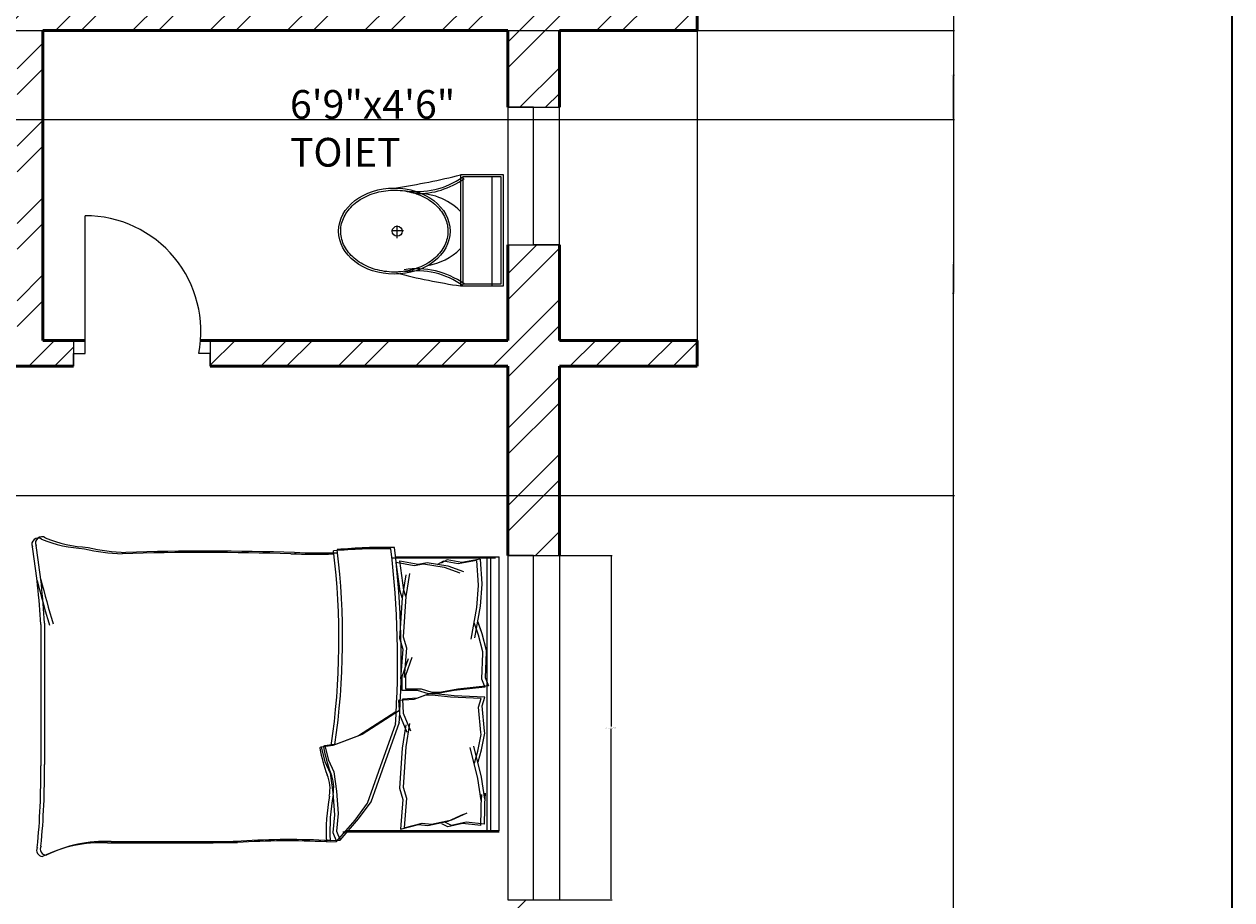
# Model space of a CAD drawing. Units: inches. Extents: x 1980 to 2738, y 1471 to 2568.
# Tile 13 of 22: x 2528 to 2738, y 1722 to 1874. Entities that reach past the tile are written whole.
import ezdxf

# ---------------------------------------------------------------- set-up
doc = ezdxf.new("R2010")
doc.units = ezdxf.units.IN
for name, color, linetype, lineweight in [('A-ANNO-DIMS', 2, 'Continuous', 18), ('A-ANNO-TTLB', 7, 'Continuous', 35), ('A-AREA-IDEN', 7, 'Continuous', 18), ('A-DOOR', 31, 'Continuous', 25), ('A-FLOR-BALC', 7, 'Continuous', 25), ('A-FLOR-FIXT', 8, 'Continuous', 25), ('A-FURN', 8, 'Continuous', 18), ('A-GLAZ', 141, 'Continuous', 18), ('A-WALL', 7, 'Continuous', 50)]:
    doc.layers.add(name, color=color, linetype=linetype, lineweight=lineweight)
doc.layers.add('A-WALL-PATT', color=9, linetype='Continuous', lineweight=13, true_color=0xd19cc7)
doc.styles.get("Standard").update_dxf_attribs({"font": 'arial.ttf'})
doc.dimstyles.get("Standard").update_dxf_attribs({"dimtxt": 0.18, "dimasz": 0.18, "dimexe": 0.18, "dimexo": 0.0625, "dimgap": 0.09, "dimtad": 0, "dimtih": 1, "dimtoh": 1, "dimdec": 4, "dimzin": 0, "dimdsep": 46, "dimtxsty": 'Standard', "dimcen": 0.09, "dimadec": 0, "dimazin": 0, "dimtfac": 1, "dimtdec": 4, "dimtofl": 0, "dimtmove": 0, "dimatfit": 3, "dimfxl": 1, "dimtolj": 1, "dimtzin": 0, "dimarcsym": 0})

# ---------------------------------------------------------------- blocks, each defined once
blk = doc.blocks.new('A$C31115884')
for p, q in [((257.5, 466.4), (257.5, 523.2)), ((283.1, 497.7), (223.4, 497.7)), ((0, 200), (0, 0)), ((520, 200), (0, 200)), ((10, 190), (10, 10)), ((510, 190), (10, 190)), ((510, 10), (510, 190)), ((520, 0), (520, 200)), ((510, 54.5), (0, 54.5)), ((10, 10), (510, 10)), ((0, 0), (520, 0))]:
    blk.add_line(p, q)
blk.add_circle((255.6, 496.4), 23.6)
for centre, radius, start, end in [((2777.7, -204.6), 2807, 165.4549, 171.7133), ((-294.5, 403.3), 364.7, 324.2091, 9.3499), ((-294.5, 403.3), 374.7, 324.2091, 9.3499), ((805.8, 403.3), 364.7, 170.6501, 215.7909), ((3237, 905), 2807, 188.2867, 194.5451), ((139.5, 406.2), 293.5, 315.8436, 2.6563), ((805.8, 403.3), 374.7, 179.2036, 215.7909), ((383.6, 406.2), 293.5, 190.2774, 224.1564)]:
    blk.add_arc(centre, radius, start, end)
blk.add_ellipse((256.2, 509.9), major_axis=(0, -260.7), ratio=0.772727)
blk.add_open_spline([(256.2, 259.2), (263.1, 259.2), (270, 259.7), (287.8, 262.3), (298.7, 265.1), (319.9, 273.1), (330.2, 278.4), (350.1, 291.1), (359.7, 298.7), (377.7, 315.9), (386.2, 325.5), (401.7, 346.6), (408.8, 358.1), (421.3, 382.5), (426.8, 395.5), (435.9, 422.4), (439.5, 436.4), (444.8, 465.1), (446.5, 479.7), (447.9, 509.2), (447.6, 524), (445, 553.3), (442.7, 567.8), (436.3, 596), (432.1, 609.7), (421.9, 636), (416, 648.6), (402.5, 672.1), (395, 683), (378.6, 703), (369.8, 712.1), (351.1, 728), (341.3, 734.8), (320.9, 746.2), (310.4, 750.7), (288.9, 757.3), (278, 759.4), (256, 761), (245, 760.6), (223.1, 757.2), (212.3, 754.3), (191.1, 746.1), (180.8, 740.7), (160.9, 727.8), (151.4, 720.1), (133.5, 702.7), (125.1, 693), (109.6, 671.7), (102.6, 660.2), (90.2, 635.7), (84.9, 622.7), (76, 595.6), (72.4, 581.6), (67.2, 552.9), (65.6, 538.2), (64.4, 508.8), (64.8, 494), (67.5, 464.7), (69.9, 450.2), (76.6, 422), (80.8, 408.3), (91.1, 382.2), (97.2, 369.7), (110.8, 346.3), (118.4, 335.4), (134.8, 315.6), (143.7, 306.7), (162.4, 290.9), (172.3, 284.2), (192.8, 273), (203.3, 268.6), (224.8, 262.2), (235.8, 260.2), (249.9, 259.3), (253, 259.2), (256.2, 259.2)], degree=3, knots=[0, 0, 0, 0, 0.110105, 0.110105, 0.285049, 0.285049, 0.459994, 0.459994, 0.634938, 0.634938, 0.809882, 0.809882, 0.984827, 0.984827, 1.159771, 1.159771, 1.334715, 1.334715, 1.50966, 1.50966, 1.684604, 1.684604, 1.859549, 1.859549, 2.034493, 2.034493, 2.209437, 2.209437, 2.384382, 2.384382, 2.559326, 2.559326, 2.73427, 2.73427, 2.909215, 2.909215, 3.084159, 3.084159, 3.259103, 3.259103, 3.434048, 3.434048, 3.608992, 3.608992, 3.783936, 3.783936, 3.958881, 3.958881, 4.133825, 4.133825, 4.30877, 4.30877, 4.483714, 4.483714, 4.658658, 4.658658, 4.833603, 4.833603, 5.008547, 5.008547, 5.183491, 5.183491, 5.358436, 5.358436, 5.53338, 5.53338, 5.708324, 5.708324, 5.883269, 5.883269, 6.058213, 6.058213, 6.233158, 6.233158, 6.283185, 6.283185, 6.283185, 6.283185])
blk = doc.blocks.new('BED-DOUBLE')
for p, q in [((27.75, 52.87), (24.5, 49.16)), ((27.75, 52.87), (24.5, 49.16)), ((28.38, 53.1), (25.13, 49.39)), ((28.38, 53.1), (25.13, 49.39)), ((29.49, 52.95), (27.75, 52.87, 3.87)), ((29.49, 52.95), (27.75, 52.87, 3.87)), ((28.36, 51.33), (27.75, 52.87)), ((28.36, 51.33), (27.75, 52.87)), ((30.13, 53.18), (28.38, 53.1, 3.87)), ((30.13, 53.18), (28.38, 53.1, 3.87)), ((29, 51.56), (28.38, 53.1)), ((29, 51.56), (28.38, 53.1)), ((0, 51.49), (0.64, 51.49)), ((0, 51.27), (26.61, 51.27)), ((0, 51.27), (26.61, 51.27)), ((0, 51.27), (0, 3.48)), ((0.64, 51.49), (27.25, 51.49)), ((0.64, 51.49), (27.25, 51.49)), ((1.53, 3.48), (1.53, 51.27)), ((1.53, 3.48), (1.53, 51.27)), ((2.17, 3.7), (2.17, 51.49)), ((2.17, 3.7), (2.17, 51.49)), ((6.41, 49.96), (8.98, 50.56)), ((6.41, 49.96), (8.98, 50.56)), ((8.98, 50.56), (10.02, 50.04)), ((8.98, 50.56), (10.02, 50.04)), ((16.57, 50.7), (13.43, 49.92)), ((16.57, 50.7), (13.43, 49.92)), ((17.21, 50.93), (14.07, 50.15)), ((17.21, 50.93), (14.07, 50.15)), ((16.17, 45.57), (16.57, 50.7)), ((16.17, 45.57), (16.57, 50.7)), ((16.81, 45.8), (17.21, 50.93)), ((16.81, 45.79), (17.21, 50.93)), ((28.06, 48.23), (28.36, 51.33)), ((28.06, 48.23), (28.36, 51.33)), ((28.69, 48.46), (29, 51.56)), ((28.69, 48.46), (29, 51.56)), ((2.56, 50.11), (2.46, 44.71)), ((2.56, 50.11), (2.46, 44.71)), ((2.56, 50.11), (5.77, 49.73)), ((2.56, 50.11), (5.77, 49.73)), ((3.2, 50.34), (3.1, 44.94)), ((3.2, 50.34), (3.1, 44.94)), ((3.2, 50.34), (6.41, 49.96)), ((3.2, 50.34), (6.41, 49.96)), ((8.26, 49.31), (5.58, 48.13)), ((8.26, 49.31), (5.58, 48.13)), ((5.77, 49.73), (8.34, 50.33)), ((5.77, 49.73), (8.34, 50.33)), ((8.9, 49.54), (6.22, 48.36)), ((8.9, 49.54), (6.22, 48.36)), ((11.83, 50.11), (8.26, 49.31)), ((11.83, 50.11), (8.26, 49.31)), ((8.34, 50.33), (9.38, 49.81)), ((8.34, 50.33), (9.38, 49.81)), ((12.47, 50.34), (8.9, 49.54)), ((12.47, 50.34), (8.9, 49.54)), ((13.43, 49.92), (11.83, 50.11)), ((13.43, 49.92), (11.83, 50.11)), ((14.07, 50.15), (12.47, 50.34)), ((14.07, 50.15), (12.47, 50.34)), ((24.5, 49.16), (22.33, 46.22)), ((24.5, 49.16), (22.33, 46.22)), ((25.13, 49.39), (22.97, 46.45)), ((25.13, 49.39), (22.97, 46.45)), ((29, 44.59), (28.69, 48.46)), ((29, 44.59), (28.69, 48.46)), ((22.97, 46.45), (20.96, 40.87)), ((22.97, 46.45), (20.96, 40.87)), ((28.36, 44.36), (28.06, 48.23)), ((28.36, 44.36), (28.06, 48.23)), ((2.46, 44.71), (2.54, 45.71)), ((2.46, 44.71), (2.54, 45.71)), ((2.54, 45.71), (3.07, 41.91)), ((2.54, 45.71), (3.07, 41.91)), ((3.1, 44.94), (3.18, 45.94)), ((3.1, 44.94), (3.18, 45.94)), ((3.18, 45.94), (3.71, 42.14)), ((3.18, 45.94), (3.71, 42.14)), ((16.73, 43.61), (16.17, 45.57)), ((16.73, 43.61), (16.17, 45.57)), ((17.37, 43.83), (16.81, 45.8)), ((17.37, 43.83), (16.81, 45.79)), ((22.33, 46.22), (20.32, 40.64)), ((22.33, 46.22), (20.32, 40.64)), ((28.83, 40.95), (28.36, 44.36)), ((28.83, 40.95), (28.36, 44.36)), ((29.47, 41.18), (29, 44.59)), ((29.47, 41.18), (29, 44.59)), ((3.71, 42.14), (5.06, 36.72)), ((3.71, 42.14), (5.06, 36.72)), ((16.29, 36.6), (16.73, 43.61)), ((16.29, 36.6), (16.73, 43.61)), ((16.93, 36.82), (17.37, 43.83)), ((16.93, 36.82), (17.37, 43.83)), ((3.07, 41.91), (4.42, 36.5)), ((3.07, 41.91), (4.42, 36.5)), ((20.32, 40.64), (17.38, 32.31)), ((20.32, 40.64), (17.38, 32.31)), ((20.96, 40.87), (18.02, 32.53)), ((20.96, 40.87), (18.02, 32.53)), ((29.76, 38.94), (28.83, 40.95)), ((29.76, 38.94), (28.83, 40.95)), ((30.4, 39.17), (29.47, 41.18)), ((30.4, 39.17), (29.47, 41.18)), ((3.67, 39.2), (3.08, 37.14)), ((3.67, 39.2), (3.08, 37.14)), ((4.31, 39.43), (3.72, 37.36)), ((4.31, 39.43), (3.72, 37.36)), ((30.38, 36.46), (29.76, 38.94)), ((30.38, 36.46), (29.76, 38.94)), ((31.02, 36.69), (30.4, 39.17)), ((31.02, 36.69), (30.4, 39.17)), ((79.24, 15.06), (79.24, 39.68)), ((79.24, 15.06), (79.24, 39.68)), ((79.88, 15.29), (79.88, 39.91)), ((79.88, 15.29), (79.88, 39.91)), ((3.08, 37.14), (2.54, 34.2)), ((3.08, 37.14), (2.54, 34.2)), ((3.72, 37.36), (3.18, 34.43)), ((3.72, 37.36), (3.18, 34.43)), ((15.63, 32.56), (16.29, 36.6)), ((15.63, 32.56), (16.29, 36.6)), ((16.27, 32.79), (16.93, 36.82)), ((16.27, 32.79), (16.93, 36.82)), ((23.88, 34.45), (28.36, 36.15)), ((23.88, 34.45), (28.36, 36.15)), ((24.52, 34.68), (29, 36.38)), ((24.52, 34.68), (29, 36.38)), ((28.36, 36.15), (30.38, 36.46)), ((28.36, 36.15), (30.38, 36.46)), ((29, 36.38), (31.02, 36.69)), ((29, 36.38), (31.02, 36.69)), ((2.54, 34.2), (2.56, 33.88)), ((2.54, 34.2), (2.56, 33.88)), ((2.56, 33.88), (2.98, 29.46)), ((2.56, 33.88), (2.98, 29.46)), ((3.18, 34.43), (3.2, 34.11)), ((3.18, 34.43), (3.2, 34.11)), ((3.2, 34.11), (3.62, 29.68)), ((3.2, 34.11), (3.62, 29.68)), ((16.74, 30.75), (15.45, 33.82)), ((16.74, 30.75), (15.45, 33.82)), ((17.38, 30.98), (16.09, 34.05)), ((17.38, 30.98), (16.09, 34.05)), ((17.38, 30.26), (23.88, 34.45)), ((17.38, 30.26), (23.88, 34.45)), ((18.02, 30.49), (24.52, 34.68)), ((18.02, 30.49), (24.52, 34.68)), ((3.62, 29.68), (3.13, 28.21)), ((3.62, 29.68), (3.13, 28.21)), ((16.89, 28.3), (16.74, 30.75)), ((16.89, 28.3), (16.74, 30.75)), ((17.53, 28.53), (17.38, 30.98)), ((17.53, 28.53), (17.38, 30.98)), ((2.98, 29.46), (2.49, 27.98)), ((2.98, 29.46), (2.49, 27.98)), ((2.49, 27.98), (7.87, 27.73)), ((2.49, 27.98), (7.87, 27.73)), ((3.13, 28.21), (8.51, 27.96)), ((3.13, 28.21), (8.51, 27.96)), ((7.86, 26.79), (11.04, 27.37)), ((7.86, 26.79), (11.04, 27.37)), ((7.87, 27.73), (11.08, 27.36)), ((7.87, 27.73), (11.08, 27.35)), ((8.51, 27.96), (11.72, 27.58)), ((8.51, 27.96), (11.72, 27.58)), ((11.04, 27.37), (12.34, 27.37)), ((11.04, 27.37), (12.34, 27.37)), ((11.08, 27.36), (12.38, 27.44)), ((11.08, 27.35), (12.38, 27.44)), ((11.72, 27.58), (13.02, 27.66)), ((11.72, 27.58), (13.02, 27.66)), ((12.34, 27.37), (14.22, 26.79)), ((12.34, 27.37), (14.22, 26.79)), ((12.38, 27.44), (14.22, 28.13)), ((12.38, 27.44), (14.22, 28.13)), ((13.02, 27.66), (14.86, 28.36)), ((13.02, 27.66), (14.86, 28.36)), ((14.22, 28.13), (16.89, 28.3)), ((14.22, 28.13), (16.89, 28.3)), ((14.86, 28.36), (17.53, 28.53)), ((14.86, 28.36), (17.53, 28.53)), ((1.87, 25.98), (7.22, 26.56)), ((1.87, 25.98), (7.22, 26.56)), ((2.45, 24.54), (1.87, 25.98)), ((2.45, 24.54), (1.87, 25.98)), ((2.51, 26.21), (7.86, 26.79)), ((2.51, 26.21), (7.86, 26.79)), ((3.09, 24.77), (2.51, 26.21)), ((3.09, 24.77), (2.51, 26.21)), ((7.22, 26.56), (10.4, 27.14)), ((7.22, 26.56), (10.4, 27.14)), ((10.4, 27.14), (11.7, 27.14)), ((10.4, 27.14), (11.7, 27.14)), ((11.7, 27.14), (13.58, 26.56)), ((11.7, 27.14), (13.58, 26.56)), ((13.58, 26.56), (16.26, 26.56)), ((13.58, 26.56), (16.26, 26.56)), ((14.22, 26.79), (16.9, 26.79)), ((14.22, 26.79), (16.9, 26.79)), ((16.26, 26.56), (16.26, 24.1)), ((16.26, 26.56), (16.26, 24.1)), ((16.9, 26.79), (16.9, 24.33)), ((16.9, 26.79), (16.9, 24.33)), ((2.3, 20.09), (2.45, 24.54)), ((2.3, 20.09), (2.45, 24.54)), ((2.94, 20.32), (3.09, 24.77)), ((2.94, 20.32), (3.09, 24.77)), ((16.26, 24.1), (15.17, 20.96)), ((16.26, 24.1), (15.17, 20.96)), ((16.9, 24.33), (15.81, 21.19)), ((16.9, 24.33), (15.81, 21.19)), ((16.17, 19.38), (16.57, 24.52)), ((16.17, 19.38), (16.57, 24.52)), ((16.81, 19.61), (17.21, 24.74)), ((16.81, 19.61), (17.21, 24.74)), ((2.3, 19.77), (2.3, 20.09)), ((2.3, 19.77), (2.3, 20.09)), ((3.03, 16.88), (2.3, 19.77)), ((3.03, 16.88), (2.3, 19.77)), ((2.94, 20), (2.94, 20.32)), ((2.94, 20), (2.94, 20.32)), ((3.67, 17.11), (2.94, 20)), ((3.67, 17.11), (2.94, 20)), ((16.73, 17.42), (16.17, 19.38)), ((16.73, 17.42), (16.17, 19.38)), ((17.37, 17.65), (16.81, 19.61)), ((17.37, 17.65), (16.81, 19.61)), ((3.75, 14.86), (3.03, 16.88)), ((3.75, 14.85), (3.03, 16.88)), ((3.32, 12.11), (4.33, 17.6)), ((3.32, 12.11), (4.33, 17.6)), ((4.39, 15.08), (3.67, 17.11)), ((4.39, 15.08), (3.67, 17.11)), ((3.96, 12.34), (4.97, 17.83)), ((3.96, 12.34), (4.97, 17.83)), ((16.29, 10.41), (16.73, 17.42)), ((16.29, 10.41), (16.73, 17.42)), ((16.93, 10.64), (17.37, 17.65)), ((16.93, 10.64), (17.37, 17.65)), ((3.03, 8.29), (3.32, 12.11)), ((3.03, 8.28), (3.32, 12.11)), ((3.67, 8.51), (3.96, 12.34)), ((3.67, 8.51), (3.96, 12.34)), ((16.27, 6.61), (16.93, 10.64)), ((16.27, 6.61), (16.93, 10.64)), ((16.93, 10.64), (17.26, 9.51)), ((16.93, 10.64), (17.26, 9.51)), ((3.65, 8.41), (3.67, 8.51)), ((3.65, 8.41), (3.67, 8.51)), ((15.63, 6.38), (16.29, 10.41)), ((15.63, 6.38), (16.29, 10.41)), ((16.29, 10.41), (16.62, 9.28)), ((16.29, 10.41), (16.62, 9.28)), ((16.62, 9.28), (17.34, 4.18)), ((16.62, 9.28), (17.34, 4.18)), ((17.26, 9.51), (17.98, 4.41)), ((17.26, 9.51), (17.98, 4.41)), ((3.01, 8.18), (3.03, 8.29)), ((3.01, 8.18), (3.03, 8.28)), ((3.34, 3.9), (3.01, 8.18)), ((3.34, 3.9), (3.01, 8.18)), ((3.98, 4.13), (3.65, 8.41)), ((3.98, 4.13), (3.65, 8.41)), ((3.32, 3.89), (6.5, 4.47)), ((3.32, 3.89), (6.5, 4.47)), ((3.96, 4.12), (7.14, 4.7)), ((3.96, 4.12), (7.14, 4.7)), ((8.95, 5.05), (6.21, 6.06)), ((8.95, 5.05), (6.21, 6.06)), ((6.5, 4.47), (9.1, 4.04)), ((6.5, 4.47), (9.1, 4.04)), ((9.59, 5.28), (6.85, 6.29)), ((9.59, 5.28), (6.85, 6.29)), ((7.14, 4.7), (9.74, 4.27)), ((7.14, 4.7), (9.74, 4.27)), ((12.57, 4.47), (8.95, 5.05)), ((12.57, 4.47), (8.95, 5.05)), ((9.1, 4.04), (10.11, 4.62)), ((9.1, 4.04), (10.11, 4.62)), ((13.21, 4.7), (9.59, 5.28)), ((13.21, 4.7), (9.59, 5.28)), ((9.74, 4.27), (10.75, 4.85)), ((9.74, 4.27), (10.75, 4.85)), ((14.16, 4.76), (12.57, 4.47)), ((14.16, 4.76), (12.57, 4.47)), ((14.8, 4.99), (13.21, 4.7)), ((14.8, 4.99), (13.21, 4.7)), ((17.34, 4.18), (14.16, 4.76)), ((17.34, 4.18), (14.16, 4.76)), ((17.98, 4.41), (14.8, 4.99)), ((17.98, 4.41), (14.8, 4.99)), ((18.11, 3.48), (0, 3.48)), ((18.11, 3.48), (0, 3.48)), ((18.75, 3.7), (0.64, 3.7)), ((18.75, 3.7), (0.64, 3.7))]:
    blk.add_line(p, q)
for centre, radius, start, end in [((68.67, 76.16), 23.07, 267.4714, 296.4681), ((68.67, 76.16), 23.07, 267.4714, 296.4681), ((69.31, 76.39), 23.07, 267.4714, 296.4681), ((69.31, 76.39), 23.07, 267.4714, 296.4681), ((78.87, 54.41), 1.1, 332.6588, 86.02), ((78.87, 54.41), 1.1, 332.6588, 86.02), ((79.51, 54.64), 1.1, 332.6588, 86.02), ((79.51, 54.64), 1.1, 332.6588, 86.02), ((-6.66, 51.33), 36.18, 349.8763, 2.5657), ((-6.66, 51.33), 36.18, 349.8763, 2.5657), ((36.31, 182.27), 129.5, 266.9791, 273.8365), ((36.31, 182.27), 129.5, 266.9791, 273.8365), ((-6.02, 51.56), 36.18, 349.8763, 2.5657), ((-6.02, 51.56), 36.18, 349.8763, 2.5657), ((36.95, 182.49), 129.5, 266.9791, 273.8365), ((36.95, 182.49), 129.5, 266.9791, 273.8365), ((67.82, -4508.74), 4561.86, 90.00217, 90.28689), ((67.82, -4508.74), 4561.86, 90.00217, 90.28689), ((68.46, -4508.51), 4561.86, 90.00217, 90.28689), ((68.46, -4508.52), 4561.86, 90.00217, 90.28689), ((212.28, 41.15), 133.04, 174.4998, 180.6351), ((212.28, 41.15), 133.04, 174.4998, 180.6351), ((212.92, 41.38), 133.04, 174.4998, 180.6351), ((212.92, 41.38), 133.04, 174.4998, 180.6351), ((35.07, 43.74), 6.22, 168.6608, 203.7384), ((35.07, 43.74), 6.22, 168.6608, 203.7384), ((35.71, 43.97), 6.22, 168.6608, 203.7384), ((35.71, 43.97), 6.22, 168.6608, 203.7384), ((1.48, 31.15), 29.65, 10.6617, 19.8806), ((1.48, 31.15), 29.65, 10.6617, 19.8806), ((2.12, 31.38), 29.65, 10.6617, 19.8806), ((2.12, 31.38), 29.65, 10.6617, 19.8806), ((156.32, 17.76), 129.02, 171.7845, 186.9006), ((156.32, 17.76), 129.02, 171.7845, 186.9006), ((156.96, 17.98), 129.02, 171.7845, 186.9006), ((156.96, 17.98), 129.02, 171.7845, 186.9006), ((30.44, 36.64), 0.185, 250.2464, 1.1377), ((30.44, 36.64), 0.185, 250.2464, 1.1377), ((31.08, 36.86), 0.185, 250.2464, 1.1377), ((31.08, 36.86), 0.185, 250.2464, 1.1377), ((182.05, 21.36), 164.97, 176.0865, 186.7821), ((182.05, 21.36), 164.97, 176.0865, 186.7821), ((182.69, 21.59), 164.97, 176.0865, 186.7821), ((182.69, 21.59), 164.97, 176.0865, 186.7821), ((-23.71, -17.22), 106.46, 13.3832, 17.7053), ((-23.71, -17.22), 106.46, 13.3832, 17.7053), ((-23.07, -16.99), 106.46, 13.3832, 17.7053), ((-23.07, -16.99), 106.46, 13.3832, 17.7053), ((200.84, 21.43), 121.76, 182.9958, 189.4091), ((200.84, 21.43), 121.76, 182.9958, 189.4091), ((201.48, 21.66), 121.76, 182.9958, 189.4091), ((201.48, 21.66), 121.76, 182.9958, 189.4091), ((20.1, 85.16), 83.31, 268.7218, 275.604), ((20.1, 85.16), 83.31, 268.7218, 275.604), ((20.74, 85.39), 83.31, 268.7218, 275.604), ((20.74, 85.39), 83.31, 268.7218, 275.604), ((31.17, -167.31), 170.11, 88.4762, 91.0082), ((31.17, -167.31), 170.11, 88.4762, 91.0082), ((31.81, -167.08), 170.11, 88.4762, 91.0082), ((31.81, -167.08), 170.11, 88.4762, 91.0082), ((50.61, 484.82), 482.31, 268.2277, 271.7185), ((50.61, 484.82), 482.31, 268.2277, 271.7185), ((51.25, 485.05), 482.31, 268.2277, 271.7185), ((51.25, 485.05), 482.31, 268.2277, 271.7185), ((64.51, -26.9), 29.63, 76.0648, 88.9113), ((64.51, -26.9), 29.63, 76.0648, 88.9113), ((65.15, -26.67), 29.63, 76.0648, 88.9113), ((65.15, -26.67), 29.63, 76.0648, 88.9113), ((70.28, -21.66), 23.56, 67.9751, 86.652), ((70.28, -21.66), 23.56, 67.9751, 86.652), ((70.91, -21.43), 23.56, 67.9751, 86.652), ((70.91, -21.43), 23.56, 67.9751, 86.652), ((79.72, 1.09), 1.09, 236.1736, 23.4781), ((79.72, 1.09), 1.09, 236.1736, 23.4781), ((80.36, 1.32), 1.09, 236.1736, 23.4781), ((80.36, 1.32), 1.09, 236.1736, 23.4781)]:
    blk.add_arc(centre, radius, start, end)
blk = doc.blocks.new('WIN-24IN-WALL')
for p, q in [((4.5, 24), (0, 24)), ((0, 24), (9, 24)), ((0, 24), (0, 0)), ((4.5, 0), (4.5, 24)), ((9, 0), (9, 24)), ((0, 0), (9, 0)), ((9, 0), (4.5, 0))]:
    blk.add_line(p, q)
blk = doc.blocks.new('WIN-60IN-WALL-SINGLE-JAMB-LINE')
for p, q in [((4.5, 60), (0, 60)), ((0, 60), (9, 60)), ((0, 60), (0, 0)), ((4.5, 0), (4.5, 60)), ((9, 60), (9, 0)), ((0, 0), (9, 0))]:
    blk.add_line(p, q)
blk = doc.blocks.new('*D29')
at = {"layer": 'A-ANNO-DIMS', "color": 0, "lineweight": -2, "transparency": 16777216}
for p, q in [((2621.15, 1781.73), (2630.26, 1781.73)), ((2630.08, 1781.55), (2630.08, 1751.92)), ((2630.08, 1721.91), (2630.08, 1751.55)), ((2621.15, 1721.73), (2630.26, 1721.73))]:
    blk.add_line(p, q, dxfattribs=at)
at = {"layer": 'A-ANNO-DIMS', "color": 0, "transparency": 16777216}
for points in [[(2630.05, 1781.55), (2630.11, 1781.55), (2630.08, 1781.73)], [(2630.05, 1721.91), (2630.11, 1721.91), (2630.08, 1721.73)]]:
    blk.add_solid(points, dxfattribs=at)
at = {"layer": 'Defpoints', "color": 0, "transparency": 16777216}
for p in [(2621.08, 1781.73), (2630.08, 1781.73), (2621.08, 1721.73)]:
    blk.add_point(p, dxfattribs=at)
at = {"layer": 'A-ANNO-DIMS', "color": 0, "transparency": 16777216, "insert": (2630.08, 1751.73), "char_height": 0.18, "attachment_point": 5}
blk.add_mtext('\\A1;WINDOW 60 TYP.', dxfattribs=at)
blk = doc.blocks.new('*D37')
at = {"layer": 'A-ANNO-DIMS', "color": 0, "lineweight": -2, "transparency": 16777216}
for p, q in [((2579.97, 2011.21), (2689.91, 2011.21)), ((2689.73, 2011.03), (2689.73, 1827.64)), ((2689.73, 1643.89), (2689.73, 1827.27)), ((2621.15, 1643.71), (2689.91, 1643.71))]:
    blk.add_line(p, q, dxfattribs=at)
at = {"layer": 'A-ANNO-DIMS', "color": 0, "transparency": 16777216}
for points in [[(2689.7, 2011.03), (2689.76, 2011.03), (2689.73, 2011.21)], [(2689.7, 1643.89), (2689.76, 1643.89), (2689.73, 1643.71)]]:
    blk.add_solid(points, dxfattribs=at)
at = {"layer": 'Defpoints', "color": 0, "transparency": 16777216}
for p in [(2579.9, 2011.21), (2689.73, 2011.21), (2621.08, 1643.71)]:
    blk.add_point(p, dxfattribs=at)
at = {"layer": 'A-ANNO-DIMS', "color": 0, "transparency": 16777216, "insert": (2689.73, 1827.46), "char_height": 0.18, "attachment_point": 5}
blk.add_mtext('\\A1;367.5', dxfattribs=at)
blk = doc.blocks.new('*D58')
at = {"layer": 'A-ANNO-DIMS', "color": 0, "lineweight": -2, "transparency": 16777216}
for p, q in [((2372.59, 1873.21), (2689.91, 1873.21)), ((2689.73, 1873.03), (2689.73, 1832.89)), ((2689.73, 1792.39), (2689.73, 1832.52)), ((2372.59, 1792.21), (2689.91, 1792.21))]:
    blk.add_line(p, q, dxfattribs=at)
at = {"layer": 'A-ANNO-DIMS', "color": 0, "transparency": 16777216}
for points in [[(2689.7, 1873.03), (2689.76, 1873.03), (2689.73, 1873.21)], [(2689.7, 1792.39), (2689.76, 1792.39), (2689.73, 1792.21)]]:
    blk.add_solid(points, dxfattribs=at)
at = {"layer": 'Defpoints', "color": 0, "transparency": 16777216}
for p in [(2372.53, 1873.21), (2689.73, 1873.21), (2372.53, 1792.21)]:
    blk.add_point(p, dxfattribs=at)
at = {"layer": 'A-ANNO-DIMS', "color": 0, "transparency": 16777216, "insert": (2689.73, 1832.71), "char_height": 0.18, "attachment_point": 5}
blk.add_mtext('\\A1;81', dxfattribs=at)
blk = doc.blocks.new('*D61')
at = {"layer": 'A-ANNO-DIMS', "color": 0, "lineweight": -2, "transparency": 16777216}
for p, q in [((2114.15, 1873.21), (2689.91, 1873.21)), ((2689.73, 1873.03), (2689.73, 1865.65)), ((2689.73, 1857.91), (2689.73, 1865.29)), ((2114.15, 1857.73), (2689.91, 1857.73))]:
    blk.add_line(p, q, dxfattribs=at)
at = {"layer": 'A-ANNO-DIMS', "color": 0, "transparency": 16777216}
for points in [[(2689.7, 1873.03), (2689.76, 1873.03), (2689.73, 1873.21)], [(2689.7, 1857.91), (2689.76, 1857.91), (2689.73, 1857.73)]]:
    blk.add_solid(points, dxfattribs=at)
at = {"layer": 'Defpoints', "color": 0, "transparency": 16777216}
for p in [(2114.08, 1873.21), (2689.73, 1873.21), (2114.08, 1857.73)]:
    blk.add_point(p, dxfattribs=at)
at = {"layer": 'A-ANNO-DIMS', "color": 0, "transparency": 16777216, "insert": (2689.73, 1865.47), "char_height": 0.18, "attachment_point": 5}
blk.add_mtext('\\A1;15.48', dxfattribs=at)

msp = doc.modelspace()

# ---------------------------------------------------------------- hatches: boundary and pattern name
at = {"layer": 'A-WALL-PATT'}
h = msp.add_hatch(dxfattribs=at)
h.set_pattern_fill('ANSI32', color=256)
h.paths.add_polyline_path([(2257.5661, 2416.2064), (2257.5661, 2420.7064), (2250.5833, 2420.7064), (2250.5833, 2462.7064), (2246.0833, 2462.7064), (2246.0833, 2420.7064), (2237.0791, 2420.7064), (2237.0791, 2411.7064), (2246.0833, 2411.7064), (2246.0833, 2291.7064), (2242.6109, 2291.7064), (2242.6109, 2287.2064), (2246.0833, 2287.2064), (2250.5833, 2287.2064), (2250.5833, 2291.7064), (2250.5833, 2411.7064), (2257.5661, 2411.7064)])
h.paths.add_polyline_path([(2387.0396, 2416.2064), (2387.0396, 2420.7064), (2367.5833, 2420.7064), (2367.5833, 2462.7064), (2358.5833, 2462.7064), (2358.5833, 2420.7064), (2329.3087, 2420.7064), (2329.3087, 2411.7064), (2358.5833, 2411.7064), (2358.5833, 2321.7275), (2358.5833, 2309.7064), (2347.3089, 2309.7064), (2293.3089, 2309.7064), (2293.3089, 2259.0771), (2297.8089, 2259.0771), (2297.8089, 2305.2064), (2347.3089, 2305.2064), (2347.3089, 2284.7412), (2351.8089, 2284.7412), (2351.8089, 2305.2064), (2372.3188, 2305.2064), (2372.3761, 2284.3899), (2377.0295, 2284.3899), (2377.0295, 2299.3058), (2377.0295, 2305.2064), (2426.5295, 2305.2064), (2426.5295, 2257.5573), (2431.0295, 2257.5573), (2431.0295, 2309.7064), (2377.0295, 2309.7064), (2367.5833, 2309.7064), (2367.5833, 2321.7275), (2367.5833, 2411.7064), (2387.0396, 2411.7064)])
h.paths.add_polyline_path([(2448.5267, 2416.2064), (2448.5267, 2420.7064), (2423.0396, 2420.7064), (2423.0396, 2411.7064), (2448.5267, 2411.7064)])
h.paths.add_polyline_path([(2130.9128, 2416.2064), (2130.9128, 2420.7064), (2105.0833, 2420.7064), (2105.0833, 2386.6942), (2114.0833, 2386.6942), (2114.0833, 2411.7064), (2130.9128, 2411.7064)])
h.paths.add_polyline_path([(2212.9478, 2420.7064), (2190.9128, 2420.7064), (2190.9128, 2411.7064), (2212.9478, 2411.7064), (2212.9478, 2416.2064)])
h.paths.add_polyline_path([(2114.0833, 2326.6942), (2105.0833, 2326.6942), (2105.0833, 2291.7064), (2081.0833, 2291.7064), (2081.0833, 2287.2064), (2105.0833, 2287.2064), (2105.0833, 2276.1935), (2114.0833, 2276.1935), (2114.0833, 2287.2064), (2166.3825, 2287.2064), (2166.3825, 2289.4564), (2166.3825, 2291.7064), (2114.0833, 2291.7064)])
h.paths.add_polyline_path([(2114.0833, 2252.1935), (2105.0833, 2252.1935), (2105.0833, 2233.2064), (2081.0833, 2233.2064), (2081.0833, 2228.7064), (2105.0833, 2228.7064), (2105.0833, 2213.4478), (2114.0833, 2213.4478), (2114.0833, 2228.7064), (2195.0833, 2228.7064), (2199.5833, 2228.7064), (2208.4455, 2228.7064), (2208.4455, 2230.9564), (2208.4455, 2233.2064), (2199.5833, 2233.2064), (2199.5833, 2287.2064), (2206.8904, 2287.2064), (2206.8904, 2289.4564), (2206.8904, 2291.7064), (2189.446, 2291.7064), (2189.446, 2289.4564), (2189.446, 2287.2064), (2195.0833, 2287.2064), (2195.0833, 2233.2064), (2114.0833, 2233.2064)])
h.paths.add_polyline_path([(2114.0833, 2153.4478), (2109.5833, 2153.4478), (2105.0833, 2153.4478), (2105.0833, 2135.2374), (2114.0833, 2135.2374)], flags=17)
h.paths.add_polyline_path([(2135.9619, 2095.4081), (2140.1805, 2095.4081), (2140.1805, 2104.2064), (2114.0833, 2104.2064), (2114.0833, 2110.3997), (2109.5833, 2110.3997), (2105.0833, 2110.3997), (2105.0833, 2104.2064), (2081.0833, 2104.2064), (2081.0833, 2099.7064), (2105.0833, 2099.7064), (2127.5416, 2099.8532), (2127.5416, 2056.9393), (2136.2133, 2056.9393)], flags=17)
h.paths.add_polyline_path([(2255.4895, 2104.2064), (2250.5833, 2104.2064), (2250.5833, 2233.2064), (2246.0833, 2233.2064), (2242.4941, 2233.2064), (2242.4941, 2228.7064), (2246.0833, 2228.7064), (2246.0833, 2104.2064), (2163.6825, 2104.2064), (2163.6825, 2099.8072), (2163.6825, 2095.4081), (2191.4325, 2095.4081), (2191.4325, 2011.2064), (2186.0833, 2011.2064), (2136.5143, 2010.8824), (2136.3702, 2032.9403), (2131.9559, 2032.9115), (2127.5416, 2032.8826), (2127.5416, 2006.7064), (2105.0833, 2006.7064), (2081.0833, 2006.7064), (2081.0833, 2002.2064), (2105.0833, 2002.2064), (2105.0833, 1995.9329), (2114.0833, 1995.9329), (2114.0833, 2002.2064), (2246.0833, 2002.2064), (2246.0833, 1877.7064), (2242.1358, 1877.7064), (2242.1358, 1873.2064), (2250.5833, 1873.2064), (2250.5833, 2002.2064), (2255.3335, 2002.2064), (2255.3335, 2011.2064), (2195.9325, 2011.2064), (2195.9325, 2095.2064), (2255.4895, 2095.2064), (2255.4895, 2099.5471)])
h.paths.add_polyline_path([(2199.5833, 1873.2064), (2209.827, 1873.2064), (2209.827, 1875.4564), (2209.827, 1877.7064), (2114.0833, 1877.7064), (2114.0833, 1890.0968), (2105.0833, 1890.0968), (2105.0833, 1877.7064), (2081.0833, 1877.7064), (2081.0833, 1873.2064), (2105.0833, 1873.2064), (2105.0833, 1857.7279), (2114.0833, 1857.7279), (2114.0833, 1873.2064), (2195.0833, 1873.2064), (2195.0833, 1819.2064), (2190.298, 1819.2064), (2190.298, 1814.7064), (2209.8976, 1814.7064), (2209.8976, 1816.9564), (2209.8976, 1819.2064), (2199.5833, 1819.2064)])
h.paths.add_polyline_path([(2114.0833, 1814.7064), (2166.2538, 1814.7064), (2166.2538, 1816.9564), (2166.2538, 1819.2064), (2114.0833, 1819.2064), (2114.0833, 1833.7279), (2109.5833, 1833.7279), (2105.0833, 1833.7279), (2105.0833, 1819.2064), (2081.0833, 1819.2064), (2081.0833, 1814.7064), (2105.0833, 1814.7064), (2105.0833, 1782.5516), (2114.0833, 1782.5516)])
h.paths.add_polyline_path([(2114.0833, 1722.5516), (2109.5833, 1722.5516), (2105.0833, 1722.5516), (2105.0833, 1685.7064), (2124.5104, 1685.7064), (2124.5104, 1690.2064), (2124.5104, 1694.7064), (2114.0833, 1694.7064)])
h.paths.add_polyline_path([(2218.8787, 1694.7064), (2184.5104, 1694.7064), (2184.5104, 1685.7064), (2218.8787, 1685.7064), (2218.8787, 1690.2064)])
h.paths.add_polyline_path([(2250.5833, 1819.2064), (2242.6431, 1819.2064), (2242.6431, 1816.9564), (2242.6431, 1814.7064), (2246.0833, 1814.7064), (2246.0833, 1694.7064), (2240.4035, 1694.7064), (2240.4035, 1690.2064), (2240.4035, 1685.7064), (2246.0833, 1685.7064), (2246.0833, 1643.7064), (2250.5833, 1643.7064), (2250.5833, 1685.7064), (2255.9859, 1685.7064), (2255.9859, 1690.2064), (2255.9859, 1694.7064), (2250.5833, 1694.7064)])
h.paths.add_polyline_path([(2297.4764, 1694.7064), (2279.3934, 1694.7064), (2279.3934, 1690.2064), (2279.3934, 1685.7064), (2297.4764, 1685.7064), (2297.4764, 1690.2064)])
h.paths.add_polyline_path([(2377.1596, 1694.7064), (2367.5833, 1694.7064), (2367.5833, 1787.7064), (2431.0295, 1787.7064), (2431.0295, 1792.2064), (2431.0295, 1849.4149), (2428.7795, 1849.4149), (2426.5295, 1849.4149), (2426.5295, 1792.2064), (2421.5833, 1792.2064), (2367.5833, 1792.2064), (2297.8089, 1792.2064), (2297.8089, 1850.2946), (2295.5589, 1850.2946), (2293.3089, 1850.2946), (2293.3089, 1792.2064), (2293.3089, 1787.7064), (2297.8089, 1787.7064), (2358.5833, 1787.7064), (2358.5833, 1694.7064), (2333.4764, 1694.7064), (2333.4764, 1685.7064), (2358.5833, 1685.7064), (2358.5833, 1643.7064), (2367.5833, 1643.7064), (2367.5833, 1685.7064), (2377.1596, 1685.7064)])
h.paths.add_polyline_path([(2442.4912, 1694.7064), (2413.1596, 1694.7064), (2413.1596, 1685.7064), (2442.4912, 1685.7064)])
h.paths.add_polyline_path([(2480.0833, 1814.7064), (2483.4816, 1814.7064), (2483.4816, 1817.9384), (2483.4816, 1819.2064), (2475.5833, 1819.2064), (2475.5833, 1694.7064), (2470.7283, 1694.7064), (2470.7283, 1685.7064), (2475.5833, 1685.7064), (2475.5833, 1643.7064), (2480.0833, 1643.7064), (2480.0833, 1685.7064), (2486.3293, 1685.7064), (2486.3293, 1690.2064), (2486.3293, 1694.7064), (2480.0833, 1694.7064)])
h.paths.add_polyline_path([(2621.0833, 1721.7349), (2612.0833, 1721.7349), (2612.0833, 1694.7064), (2586.1453, 1694.7064), (2586.1453, 1685.7064), (2621.0833, 1685.7064)])
h.paths.add_polyline_path([(2526.1453, 1690.2064), (2526.1453, 1694.7064), (2511.584, 1694.7064), (2511.584, 1690.2064), (2511.584, 1685.7064), (2526.1453, 1685.7064)])
h.paths.add_polyline_path([(2645.0833, 1819.2064), (2621.0833, 1819.2064), (2621.0833, 1835.8527), (2616.5833, 1835.8527), (2612.0833, 1835.8527), (2612.0833, 1819.2064), (2560.2541, 1819.2064), (2560.2541, 1814.7064), (2612.0833, 1814.7064), (2612.0833, 1781.7349), (2621.0833, 1781.7349), (2621.0833, 1814.7064), (2645.0833, 1814.7064)])
h.paths.add_polyline_path([(2645.0833, 1877.7064), (2621.0833, 1877.7064), (2621.0833, 1886.4375), (2612.0833, 1886.4375), (2612.0833, 1877.7064), (2517.1032, 1877.7064), (2517.1032, 1875.4564), (2517.1032, 1873.2064), (2526.5833, 1873.2064), (2526.5833, 1819.2064), (2516.6454, 1819.2064), (2516.6454, 1816.9564), (2516.6454, 1814.7064), (2536.4445, 1814.7064), (2536.4445, 1816.9564), (2536.4445, 1819.2064), (2531.0833, 1819.2064), (2531.0833, 1873.2064), (2612.0833, 1873.2064), (2612.0833, 1859.8527), (2621.0833, 1859.8527), (2621.0833, 1873.2064), (2645.0833, 1873.2064)])
h.paths.add_polyline_path([(2645.0833, 2006.7064), (2621.0833, 2006.7064), (2588.5085, 2006.7064), (2588.5085, 2052.9125), (2579.9045, 2052.9125), (2579.9045, 2011.2064), (2519.9045, 2011.2064), (2519.9045, 2095.2064), (2553.1204, 2095.2064), (2553.1204, 2104.2064), (2480.0833, 2104.2064), (2480.0833, 2228.7064), (2484.3832, 2228.7064), (2484.3832, 2230.9564), (2484.3832, 2233.2064), (2475.5833, 2233.2064), (2475.5833, 2104.2064), (2463.1308, 2104.2064), (2463.1308, 2095.2064), (2501.2463, 2095.2064), (2510.9045, 2095.2064), (2515.4045, 2095.2064), (2515.4045, 2011.2064), (2510.9045, 2011.2064), (2501.2463, 2011.2064), (2462.5957, 2011.2064), (2462.5957, 2002.2064), (2475.5833, 2002.2064), (2475.5833, 1873.2064), (2483.6146, 1873.2064), (2483.6146, 1875.4564), (2483.6146, 1877.7064), (2480.0833, 1877.7064), (2480.0833, 2002.2064), (2612.0833, 2002.2064), (2612.0833, 1996.309), (2621.0833, 1996.309), (2621.0833, 2002.2064), (2645.0833, 2002.2064)])
h.paths.add_polyline_path([(2588.5085, 2099.7277), (2621.0833, 2099.7277), (2645.0833, 2099.7064), (2645.0833, 2104.2064), (2621.0833, 2104.2064), (2621.0833, 2109.0038), (2616.5833, 2109.0038), (2612.0833, 2109.0038), (2612.0833, 2104.2064), (2575.0621, 2104.2064), (2575.0621, 2099.7064), (2575.0621, 2095.2064), (2579.9045, 2095.2064), (2579.9045, 2076.9125), (2588.5085, 2076.9125)], flags=17)
h.paths.add_polyline_path([(2367.5833, 2002.2064), (2373.7228, 2002.2064), (2373.7228, 2006.7064), (2373.7228, 2011.2064), (2350.7889, 2011.2064), (2350.7889, 2006.7064), (2350.7889, 2002.2064), (2358.5833, 2002.2064), (2358.5833, 1877.7064), (2293.3089, 1877.7064), (2293.3089, 1870.4987), (2297.8089, 1870.4987), (2297.8089, 1873.2064), (2347.3089, 1873.2064), (2347.3089, 1847.2208), (2351.8089, 1847.2208), (2351.8089, 1873.2064), (2372.5295, 1873.2064), (2372.5295, 1847.8619), (2377.0295, 1847.8619), (2377.0295, 1873.2064), (2426.5295, 1873.2064), (2426.5295, 1868.7339), (2431.0295, 1868.7339), (2431.0295, 1877.7064), (2367.5833, 1877.7064)])
h.paths.add_polyline_path([(2531.0833, 2287.2064), (2534.2285, 2287.2064), (2534.2285, 2291.7064), (2516.7886, 2291.7064), (2516.7886, 2287.2064), (2526.5833, 2287.2064), (2526.5833, 2233.2064), (2517.9112, 2233.2064), (2517.9112, 2230.9564), (2517.9112, 2228.7064), (2526.5833, 2228.7064), (2531.0833, 2228.7064), (2612.0833, 2228.7064), (2612.0833, 2206.8504), (2621.0833, 2206.8504), (2621.0833, 2228.7064), (2645.0833, 2228.7064), (2645.0833, 2233.2064), (2621.0833, 2233.2064), (2621.0833, 2241.8536), (2616.5833, 2241.8536), (2612.0833, 2241.8536), (2612.0833, 2233.2064), (2531.0833, 2233.2064)])
h.paths.add_polyline_path([(2645.0833, 2291.7064), (2621.0833, 2291.7064), (2621.0833, 2323.0138), (2616.5833, 2323.0138), (2612.0833, 2323.0138), (2612.0833, 2291.7064), (2559.6852, 2291.7064), (2559.6852, 2289.4564), (2559.6852, 2287.2064), (2612.0833, 2287.2064), (2612.0833, 2265.8536), (2621.0833, 2265.8536), (2621.0833, 2287.2064), (2645.0833, 2287.2064)])
h.paths.add_polyline_path([(2621.0833, 2420.7064), (2582.8189, 2420.7064), (2582.8189, 2411.7064), (2612.0833, 2411.7064), (2612.0833, 2383.0138), (2621.0833, 2383.0138)])
h.paths.add_polyline_path([(2480.0833, 2411.7064), (2485.7342, 2411.7064), (2485.7342, 2416.2064), (2485.7342, 2420.7064), (2480.0833, 2420.7064), (2480.0833, 2462.7064), (2475.5833, 2462.7064), (2475.5833, 2420.7064), (2469.4083, 2420.7064), (2469.4083, 2411.7064), (2475.5833, 2411.7064), (2475.5833, 2291.7064), (2475.5833, 2287.2064), (2482.9195, 2287.2064), (2482.9195, 2289.4564), (2482.9195, 2291.7064), (2480.0833, 2291.7064)])
h.paths.add_polyline_path([(2367.5833, 2228.7064), (2431.0295, 2228.7064), (2431.0295, 2233.2064), (2431.0295, 2237.4203), (2428.7795, 2237.4203), (2426.5295, 2237.4203), (2426.5295, 2233.2064), (2377.0295, 2233.2064), (2377.0295, 2260.3837), (2372.4423, 2260.3837), (2372.517, 2233.2635), (2351.8089, 2233.2064), (2351.8089, 2260.7412), (2347.3089, 2260.7412), (2347.3089, 2233.2064), (2297.8089, 2233.2064), (2297.8089, 2236.9324), (2293.3089, 2236.9324), (2293.3089, 2228.7064), (2358.5833, 2228.7064), (2358.5833, 2104.2064), (2353.3665, 2104.2064), (2353.3665, 2095.2064), (2373.8869, 2095.2064), (2373.8869, 2099.7064), (2373.8869, 2104.2064), (2367.5833, 2104.2064)])
h.paths.add_polyline_path([(2321.2323, 2104.2064), (2303.4895, 2104.2064), (2303.4895, 2095.2064), (2321.2323, 2095.2064), (2321.2323, 2099.7064)], flags=0)
h.paths.add_polyline_path([(2415.1308, 2099.7064), (2415.1308, 2104.2064), (2404.81, 2104.2064), (2404.81, 2095.2064), (2415.1308, 2095.2064)], flags=17)
h.paths.add_polyline_path([(2318.6336, 2011.2064), (2303.3335, 2011.2064), (2303.3335, 2002.2064), (2318.6336, 2002.2064)], flags=0)
h.paths.add_polyline_path([(2414.5957, 2011.2064), (2406.2461, 2011.2064), (2406.2461, 2006.7064), (2406.2461, 2002.2064), (2414.5957, 2002.2064)], flags=17)

# ---------------------------------------------------------------- linework, layer by layer
at = {"layer": 'A-ANNO-TTLB'}
msp.add_lwpolyline([(1979.5621, 2567.5568), (2738.2543, 2567.5568), (2738.2543, 1471.317), (1979.5621, 1471.317)], close=True, dxfattribs=at)
at = {"layer": 'A-DOOR'}
for p, q in [((2538.4445, 1816.9564), (2538.4445, 1840.9564)), ((2536.4445, 1819.2064), (2536.4445, 1814.7064)), ((2560.2541, 1819.2064), (2560.2541, 1814.7064)), ((2536.4445, 1814.7064), (2536.4445, 1816.9564)), ((2536.4445, 1816.9564), (2538.4445, 1816.9564)), ((2560.2541, 1816.9564), (2558.2541, 1816.9564)), ((2560.2541, 1814.7064), (2560.2541, 1816.9564))]:
    msp.add_line(p, q, dxfattribs=at)
msp.add_arc((2538.4445, 1820.781), 20.1754, 349.072349, 90, dxfattribs=at)
at = {"layer": 'A-FLOR-BALC'}
msp.add_line((2645.0833, 2287.2064), (2645.0833, 1819.2064), dxfattribs=at)
at = {"layer": 'A-GLAZ'}
for p, q in [((2612.0833, 1835.8527), (2612.0833, 1835.8527)), ((2612.0833, 1781.7349), (2612.0833, 1781.7349))]:
    msp.add_line(p, q, dxfattribs=at)
at = {"layer": 'A-WALL'}
for p, q in [((2645.0833, 1877.7064), (2645.0833, 1873.2064)), ((2612.0833, 1873.2064), (2531.0833, 1873.2064)), ((2531.0833, 1819.2064), (2531.0833, 1873.2064)), ((2612.0833, 1873.2064), (2612.0833, 1859.8527)), ((2645.0833, 1873.2064), (2621.0833, 1873.2064)), ((2621.0833, 1873.2064), (2621.0833, 1859.8527)), ((2612.0833, 1835.8527), (2612.0833, 1819.2064)), ((2621.0833, 1835.8527), (2621.0833, 1819.2064)), ((2538.4445, 1819.2064), (2531.0833, 1819.2064)), ((2538.4445, 1819.2064), (2531.0833, 1819.2064)), ((2612.0833, 1819.2064), (2558.5584, 1819.2064)), ((2612.0833, 1819.2064), (2558.5584, 1819.2064)), ((2612.0833, 1819.2064), (2612.0833, 1819.2064)), ((2612.0833, 1819.2064), (2612.0833, 1819.2064)), ((2612.0833, 1819.2064), (2612.0833, 1819.2064)), ((2621.0833, 1819.2064), (2645.0833, 1819.2064)), ((2645.0833, 1814.7064), (2645.0833, 1819.2064)), ((2536.4445, 1814.7064), (2514.9106, 1814.7064)), ((2612.0833, 1814.7064), (2560.2541, 1814.7064)), ((2612.0833, 1814.7064), (2612.0833, 1781.7349)), ((2621.0833, 1814.7064), (2645.0833, 1814.7064)), ((2621.0833, 1814.7064), (2621.0833, 1781.7349))]:
    msp.add_line(p, q, dxfattribs=at)

# ---------------------------------------------------------------- block references
at = {"layer": 'A-FLOR-FIXT', "xscale": 0.0372717239612423, "yscale": 0.0372717239612423, "zscale": 0.0372717239612423, "rotation": 89.99999999999999}
msp.add_blockref('A$C31115884', (2611.3312, 1828.717), dxfattribs=at)
at = {"layer": 'A-FURN', "rotation": 180}
msp.add_blockref('BED-DOUBLE', (2610.6075, 1785.0069), dxfattribs=at)
at = {"layer": 'A-GLAZ'}
for name, p in [('WIN-24IN-WALL', (2612.083, 1835.8531)), ('WIN-60IN-WALL-SINGLE-JAMB-LINE', (2612.083, 1721.735))]:
    msp.add_blockref(name, p, dxfattribs=at)

# ---------------------------------------------------------------- texts
at = {"layer": 'A-AREA-IDEN', "insert": (2574.1408, 1862.8451), "char_height": 5, "attachment_point": 1}
msp.add_mtext_dynamic_manual_height_columns('6\'9"x4\'6"\\PTOIET', width=64.199081, gutter_width=12.5, heights=[0], dxfattribs=at)

# ---------------------------------------------------------------- dimensions: what is measured, and where the dimension line sits
at = {"layer": 'A-ANNO-DIMS'}
for base, p1, p2, override, picture, middle in [((2689.7333, 2011.2064), (2621.0833, 1643.7064), (2579.9045, 2011.2064), {"dimdec": 1, "dimlfac": 1, "dimrnd": 0, "dimzin": 0, "dimdsep": 46, "dimlunit": 2}, '*D37', (2689.7333, 1827.4564)), ((2689.7333, 1873.2064), (2114.0833, 1857.7279), (2114.0833, 1873.2064), {"dimdec": 2, "dimlfac": 1, "dimrnd": 0, "dimzin": 0, "dimdsep": 46, "dimlunit": 2}, '*D61', (2689.7333, 1865.4672)), ((2689.7333, 1873.2064), (2372.5295, 1792.2064), (2372.5295, 1873.2064), {"dimdec": 0, "dimlfac": 1, "dimrnd": 0, "dimzin": 0, "dimdsep": 46, "dimlunit": 2}, '*D58', (2689.7333, 1832.7064))]:
    dim = msp.add_linear_dim(base=base, p1=p1, p2=p2, angle=90, dimstyle='Standard', override=override, dxfattribs=at)
    dim.commit()
    dim.dimension.update_dxf_attribs({"geometry": picture, "text_midpoint": middle})
dim = msp.add_linear_dim(base=(2630.0833, 1781.7349), p1=(2621.0833, 1721.7349), p2=(2621.0833, 1781.7349), angle=90, text='WINDOW <> TYP.', dimstyle='Standard', override={"dimdec": 0, "dimlfac": 1, "dimrnd": 0, "dimzin": 0, "dimdsep": 46, "dimlunit": 2}, dxfattribs=at)
dim.commit()
dim.dimension.update_dxf_attribs({"geometry": '*D29', "text_midpoint": (2630.0833, 1751.7349)})

doc.saveas('drawing.dxf')
